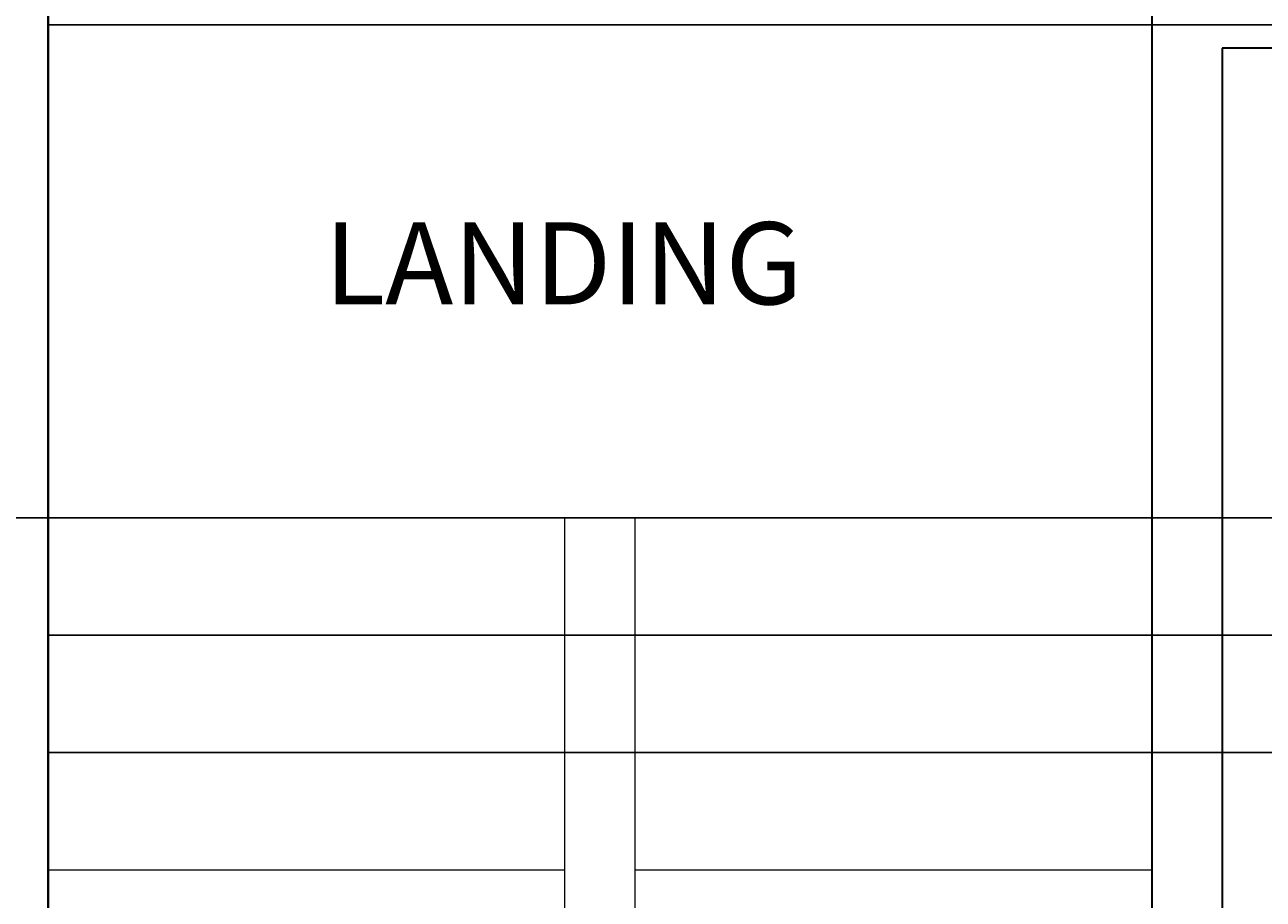
# Model space of a CAD drawing. Units: feet. Extents: x 105 to 1094, y -88 to 588.
# Tile 44 of 59: x 551 to 656, y 363 to 437. Entities that reach past the tile are written whole.
import ezdxf

# ---------------------------------------------------------------- set-up
doc = ezdxf.new("R2010")
doc.units = ezdxf.units.FT
doc.header["$MEASUREMENT"] = 0
for name, color, linetype, lineweight in [('A-ANNO-DIMS', 2, 'Continuous', 18), ('A-AREA-IDEN', 7, 'Continuous', 18), ('A-FLOR-STRS', 3, 'Continuous', 18), ('A-WALL', 7, 'Continuous', 35)]:
    doc.layers.add(name, color=color, linetype=linetype, lineweight=lineweight)
doc.styles.get("Standard").update_dxf_attribs({"font": 'arial.ttf'})
doc.dimstyles.get("Standard").update_dxf_attribs({"dimtxt": 0.18, "dimasz": 0.18, "dimexe": 0.18, "dimexo": 0.0625, "dimgap": 0.09, "dimtad": 0, "dimtih": 1, "dimtoh": 1, "dimdec": 4, "dimzin": 0, "dimdsep": 46, "dimtxsty": 'Standard', "dimcen": 0.09, "dimadec": 0, "dimazin": 0, "dimtfac": 1, "dimtdec": 4, "dimtofl": 0, "dimtmove": 0, "dimatfit": 3, "dimfxl": 1, "dimtolj": 1, "dimtzin": 0, "dimarcsym": 0})

# ---------------------------------------------------------------- blocks, each defined once
blk = doc.blocks.new('*D21')
at = {"layer": 'A-ANNO-DIMS', "color": 0, "lineweight": -2, "transparency": 16777216}
for p, q in [((849.63, 543.08), (105.46, 543.08)), ((105.64, 542.9), (105.64, 250.26)), ((105.64, -42.74), (105.64, 249.9)), ((849.63, -42.92), (105.46, -42.92))]:
    blk.add_line(p, q, dxfattribs=at)
at = {"layer": 'A-ANNO-DIMS', "color": 0, "transparency": 16777216}
for points in [[(105.61, 542.9), (105.67, 542.9), (105.64, 543.08)], [(105.61, -42.74), (105.67, -42.74), (105.64, -42.92)]]:
    blk.add_solid(points, dxfattribs=at)
at = {"layer": 'Defpoints', "color": 0, "transparency": 16777216}
for p in [(105.64, 543.08), (849.69, 543.08), (849.69, -42.92)]:
    blk.add_point(p, dxfattribs=at)
at = {"layer": 'A-ANNO-DIMS', "color": 0, "transparency": 16777216, "insert": (105.64, 250.08), "char_height": 0.18, "attachment_point": 5}
blk.add_mtext('\\A1;586', dxfattribs=at)
blk = doc.blocks.new('*D33')
at = {"layer": 'A-ANNO-DIMS', "color": 0, "lineweight": -2, "transparency": 16777216}
for p, q in [((646.63, 395.08), (105.46, 395.08)), ((105.64, 394.9), (105.64, 345.26)), ((105.64, 295.26), (105.64, 344.9)), ((646.63, 295.08), (105.46, 295.08))]:
    blk.add_line(p, q, dxfattribs=at)
at = {"layer": 'A-ANNO-DIMS', "color": 0, "transparency": 16777216}
for points in [[(105.61, 394.9), (105.67, 394.9), (105.64, 395.08)], [(105.61, 295.26), (105.67, 295.26), (105.64, 295.08)]]:
    blk.add_solid(points, dxfattribs=at)
at = {"layer": 'Defpoints', "color": 0, "transparency": 16777216}
for p in [(646.69, 395.08), (105.64, 295.08), (646.69, 295.08)]:
    blk.add_point(p, dxfattribs=at)
at = {"layer": 'A-ANNO-DIMS', "color": 0, "transparency": 16777216, "insert": (105.64, 345.08), "char_height": 0.18, "attachment_point": 5}
blk.add_mtext('\\A1;100', dxfattribs=at)
blk = doc.blocks.new('*D45')
at = {"layer": 'A-ANNO-DIMS', "color": 0, "lineweight": -2, "transparency": 16777216}
for p, q in [((552.75, 437.08), (1093.92, 437.08)), ((1093.74, 436.9), (1093.74, 416.26)), ((1093.74, 395.26), (1093.74, 415.9)), ((552.75, 395.08), (1093.92, 395.08))]:
    blk.add_line(p, q, dxfattribs=at)
at = {"layer": 'A-ANNO-DIMS', "color": 0, "transparency": 16777216}
for points in [[(1093.71, 436.9), (1093.77, 436.9), (1093.74, 437.08)], [(1093.71, 395.26), (1093.77, 395.26), (1093.74, 395.08)]]:
    blk.add_solid(points, dxfattribs=at)
at = {"layer": 'Defpoints', "color": 0, "transparency": 16777216}
for p in [(552.69, 437.08), (552.69, 395.08), (1093.74, 395.08)]:
    blk.add_point(p, dxfattribs=at)
at = {"layer": 'A-ANNO-DIMS', "color": 0, "transparency": 16777216, "insert": (1093.74, 416.08), "char_height": 0.18, "attachment_point": 5}
blk.add_mtext('\\A1;42', dxfattribs=at)
blk = doc.blocks.new('*D50')
at = {"layer": 'A-ANNO-DIMS', "color": 0, "lineweight": -2, "transparency": 16777216}
for p, q in [((552.75, 385.08), (1093.92, 385.08)), ((1093.74, 384.9), (1093.74, 380.26)), ((1093.74, 375.26), (1093.74, 379.9)), ((552.75, 375.08), (1093.92, 375.08))]:
    blk.add_line(p, q, dxfattribs=at)
at = {"layer": 'A-ANNO-DIMS', "color": 0, "transparency": 16777216}
for points in [[(1093.71, 384.9), (1093.77, 384.9), (1093.74, 385.08)], [(1093.71, 375.26), (1093.77, 375.26), (1093.74, 375.08)]]:
    blk.add_solid(points, dxfattribs=at)
at = {"layer": 'Defpoints', "color": 0, "transparency": 16777216}
for p in [(552.69, 385.08), (552.69, 375.08), (1093.74, 375.08)]:
    blk.add_point(p, dxfattribs=at)
at = {"layer": 'A-ANNO-DIMS', "color": 0, "transparency": 16777216, "insert": (1093.74, 380.08), "char_height": 0.18, "attachment_point": 5}
blk.add_mtext('\\A1;10', dxfattribs=at)

msp = doc.modelspace()

# ---------------------------------------------------------------- linework, layer by layer
at = {"layer": 'A-FLOR-STRS'}
for p, q in [((552.6883, 395.0812), (602.6883, 395.0812)), ((596.6883, 295.0812), (596.6883, 395.0812)), ((602.6883, 295.0812), (602.6883, 395.0812)), ((602.6883, 395.0812), (646.6883, 395.0812)), ((552.6883, 385.0812), (596.6883, 385.0812)), ((602.6883, 385.0812), (646.6883, 385.0812)), ((552.6883, 375.0812), (596.6883, 375.0812)), ((602.6883, 375.0812), (646.6883, 375.0812)), ((552.6883, 365.0812), (596.6883, 365.0812)), ((602.6883, 365.0812), (646.6883, 365.0812))]:
    msp.add_line(p, q, dxfattribs=at)
at = {"layer": 'A-WALL'}
for p, q in [((552.6883, 295.0812), (552.6883, 441.0812)), ((552.6883, 441.0812), (552.6883, 288.0812)), ((646.6883, 441.0812), (646.6883, 288.0812)), ((652.6883, 435.0812), (652.6883, 288.0812)), ((762.6883, 435.0812), (652.6883, 435.0812))]:
    msp.add_line(p, q, dxfattribs=at)

# ---------------------------------------------------------------- texts
at = {"layer": 'A-AREA-IDEN', "insert": (547.4026, 420.2541), "char_height": 7, "attachment_point": 1}
msp.add_mtext_dynamic_manual_height_columns('\\pxqc;LANDING ', width=98.34246, gutter_width=1, heights=[0], dxfattribs=at)

# ---------------------------------------------------------------- dimensions: what is measured, and where the dimension line sits
at = {"layer": 'A-ANNO-DIMS'}
for base, p1, p2, picture, middle in [((105.6383, 543.0812), (849.6883, -42.9188), (849.6883, 543.0812), '*D21', (105.6383, 250.0812)), ((1093.7383, 395.0812), (552.6883, 437.0812), (552.6883, 395.0812), '*D45', (1093.7383, 416.0812)), ((105.6383, 295.0812), (646.6883, 395.0812), (646.6883, 295.0812), '*D33', (105.6383, 345.0812)), ((1093.7383, 375.0812), (552.6883, 385.0812), (552.6883, 375.0812), '*D50', (1093.7383, 380.0812))]:
    dim = msp.add_linear_dim(base=base, p1=p1, p2=p2, angle=90, dimstyle='Standard', override={"dimdec": 0, "dimlfac": 1, "dimrnd": 0, "dimzin": 0, "dimdsep": 46, "dimlunit": 2}, dxfattribs=at)
    dim.commit()
    dim.dimension.update_dxf_attribs({"geometry": picture, "text_midpoint": middle})

doc.saveas('drawing.dxf')
